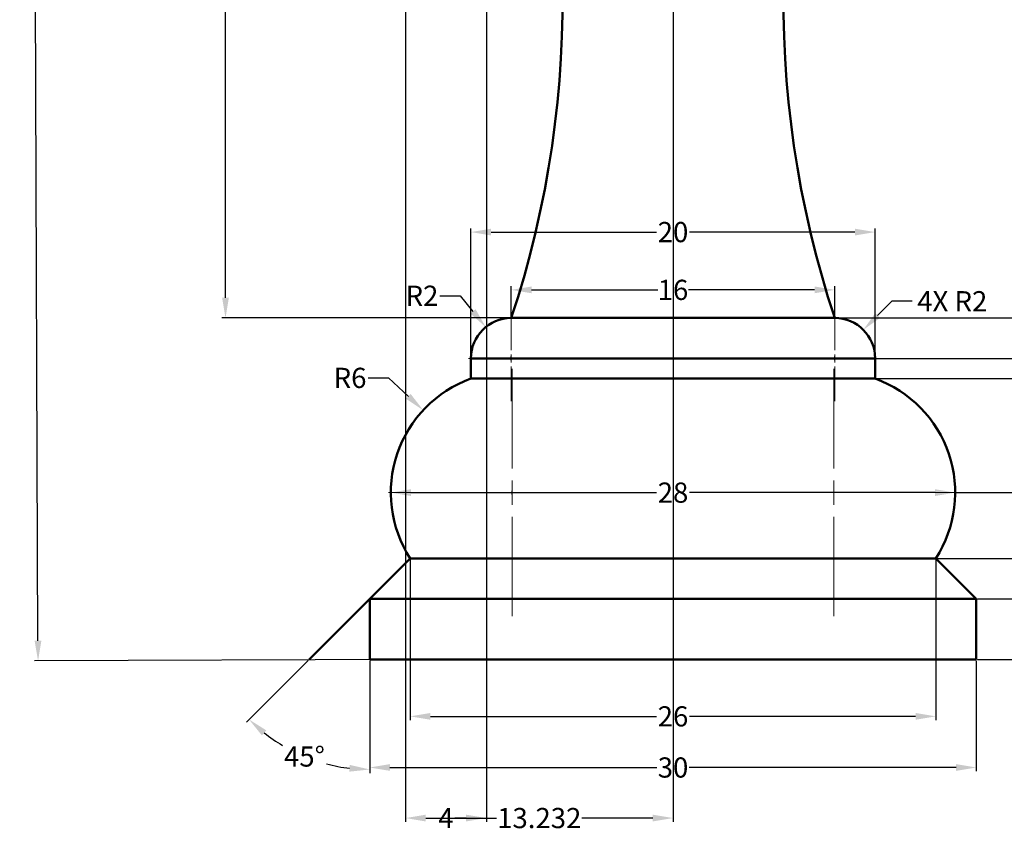
# Model space of a CAD drawing. Units: millimetres. Extents: x 31 to 232, y 35 to 192.
# Tile 1 of 5: x 31 to 80, y 35 to 75. Entities that reach past the tile are written whole.
import ezdxf

# ---------------------------------------------------------------- set-up
doc = ezdxf.new("R2010")
doc.units = ezdxf.units.MM
doc.header["$MEASUREMENT"] = 0
doc.linetypes.add('CENTER', pattern=[50.8, 31.75, -6.35, 6.35, -6.35])
for name, color, linetype, lineweight in [('M-CNTR', 1, 'CENTER', 18), ('M-DIMS', 2, 'Continuous', 25), ('M-OUTL', 7, 'Continuous', 50)]:
    doc.layers.add(name, color=color, linetype=linetype, lineweight=lineweight)
doc.styles.get("Standard").update_dxf_attribs({"font": 'arial.ttf'})
doc.dimstyles.get("Standard").update_dxf_attribs({"dimtxt": 1, "dimasz": 1, "dimexe": 0.18, "dimexo": 0.0625, "dimgap": 0.09, "dimtad": 0, "dimtih": 1, "dimtoh": 1, "dimdec": 0, "dimzin": 0, "dimdsep": 46, "dimtxsty": 'Standard', "dimcen": 0.09, "dimadec": 0, "dimazin": 0, "dimtfac": 1, "dimtdec": 0, "dimtofl": 0, "dimtmove": 0, "dimatfit": 3, "dimfxl": 1, "dimtolj": 1, "dimtzin": 0, "dimarcsym": 0})

# ---------------------------------------------------------------- blocks, each defined once
blk = doc.blocks.new('*D1')
at = {"layer": 'Defpoints', "color": 0, "transparency": 16777216}
for p in [(50.774, 48.183), (48.774, 46.183), (45.774, 43.183), (48.774, 43.183), (44.551, 38.869)]:
    blk.add_point(p, dxfattribs=at)
at = {"layer": 'M-DIMS', "color": 0, "lineweight": -2, "transparency": 16777216}
for p, q in [((45.729, 43.139), (42.674, 40.084)), ((48.774, 43.12), (48.774, 37.557))]:
    blk.add_line(p, q, dxfattribs=at)
for start, end in [(231.788, 239.2119), (255.3151, 263.212)]:
    blk.add_arc((48.774, 46.183), 8.446, start, end, dxfattribs=at)
at = {"layer": 'M-DIMS', "color": 0, "transparency": 16777216}
for points in [[(43.439, 39.422), (43.66, 39.671), (42.802, 40.211)], [(47.785, 37.963), (47.765, 37.63), (48.774, 37.737)]]:
    blk.add_solid(points, dxfattribs=at)
at = {"layer": 'M-DIMS', "color": 0, "transparency": 16777216, "insert": (45.542, 38.38), "char_height": 1, "attachment_point": 5}
blk.add_mtext('\\A1;45°', dxfattribs=at)
blk = doc.blocks.new('*D2')
at = {"layer": 'Defpoints', "color": 0, "transparency": 16777216}
for p in [(51.415, 55.522), (55.813, 51.44)]:
    blk.add_point(p, dxfattribs=at)
at = {"layer": 'M-DIMS', "color": 0, "lineweight": -2, "transparency": 16777216}
for p, q in [((48.694, 57.119), (49.694, 57.119)), ((49.694, 57.119), (50.682, 56.202)), ((55.723, 51.44), (55.903, 51.44)), ((55.813, 51.35), (55.813, 51.53))]:
    blk.add_line(p, q, dxfattribs=at)
at = {"layer": 'M-DIMS', "color": 0, "transparency": 16777216}
blk.add_solid([(50.795, 56.324), (50.568, 56.08), (51.415, 55.522)], dxfattribs=at)
at = {"layer": 'M-DIMS', "color": 0, "transparency": 16777216, "insert": (47.798, 57.119), "char_height": 1, "attachment_point": 5}
blk.add_mtext('\\A1;R6', dxfattribs=at)
blk = doc.blocks.new('*D3')
at = {"layer": 'Defpoints', "color": 0, "transparency": 16777216}
for p in [(54.51, 59.633), (55.774, 58.083)]:
    blk.add_point(p, dxfattribs=at)
at = {"layer": 'M-DIMS', "color": 0, "lineweight": -2, "transparency": 16777216}
for p, q in [((52.247, 61.184), (53.247, 61.184)), ((53.247, 61.184), (53.878, 60.408)), ((55.684, 58.083), (55.864, 58.083)), ((55.774, 57.993), (55.774, 58.173))]:
    blk.add_line(p, q, dxfattribs=at)
at = {"layer": 'M-DIMS', "color": 0, "transparency": 16777216}
blk.add_solid([(54.008, 60.514), (53.749, 60.303), (54.51, 59.633)], dxfattribs=at)
at = {"layer": 'M-DIMS', "color": 0, "transparency": 16777216, "insert": (51.356, 61.184), "char_height": 1, "attachment_point": 5}
blk.add_mtext('\\A1;R2', dxfattribs=at)
blk = doc.blocks.new('*D4')
at = {"layer": 'Defpoints', "color": 0, "transparency": 16777216}
for p in [(78.774, 46.183), (119.423, 46.183), (78.774, 43.183)]:
    blk.add_point(p, dxfattribs=at)
at = {"layer": 'M-DIMS', "color": 0, "lineweight": -2, "transparency": 16777216}
for p, q in [((119.423, 46.183), (119.423, 47.183)), ((119.423, 47.183), (120.423, 47.183)), ((78.836, 46.183), (119.603, 46.183)), ((119.423, 44.183), (119.423, 45.183)), ((78.836, 43.183), (119.603, 43.183))]:
    blk.add_line(p, q, dxfattribs=at)
at = {"layer": 'M-DIMS', "color": 0, "transparency": 16777216}
for points in [[(119.256, 45.183), (119.589, 45.183), (119.423, 46.183)], [(119.256, 44.183), (119.589, 44.183), (119.423, 43.183)]]:
    blk.add_solid(points, dxfattribs=at)
at = {"layer": 'M-DIMS', "color": 0, "transparency": 16777216, "insert": (120.84, 47.183), "char_height": 1, "attachment_point": 5}
blk.add_mtext('\\A1;3', dxfattribs=at)
blk = doc.blocks.new('*D5')
at = {"layer": 'Defpoints', "color": 0, "transparency": 16777216}
for p in [(76.774, 48.183), (119.423, 48.183), (78.774, 46.183)]:
    blk.add_point(p, dxfattribs=at)
at = {"layer": 'M-DIMS', "color": 0, "lineweight": -2, "transparency": 16777216}
for p, q in [((119.423, 49.183), (119.423, 50.183)), ((76.836, 48.183), (119.603, 48.183)), ((78.836, 46.183), (119.603, 46.183)), ((119.423, 45.183), (119.423, 44.183))]:
    blk.add_line(p, q, dxfattribs=at)
at = {"layer": 'M-DIMS', "color": 0, "transparency": 16777216}
for points in [[(119.256, 49.183), (119.589, 49.183), (119.423, 48.183)], [(119.256, 45.183), (119.589, 45.183), (119.423, 46.183)]]:
    blk.add_solid(points, dxfattribs=at)
at = {"layer": 'M-DIMS', "color": 0, "transparency": 16777216, "insert": (119.423, 47.183), "char_height": 1, "attachment_point": 5}
blk.add_mtext('\\A1;2', dxfattribs=at)
blk = doc.blocks.new('*D6')
at = {"layer": 'Defpoints', "color": 0, "transparency": 16777216}
for p in [(77.735, 51.44), (119.423, 51.44), (76.774, 48.183)]:
    blk.add_point(p, dxfattribs=at)
at = {"layer": 'M-DIMS', "color": 0, "lineweight": -2, "transparency": 16777216}
for p, q in [((119.423, 51.44), (119.423, 52.44)), ((119.423, 52.44), (120.423, 52.44)), ((77.797, 51.44), (119.603, 51.44)), ((119.423, 49.183), (119.423, 50.44)), ((76.836, 48.183), (119.603, 48.183))]:
    blk.add_line(p, q, dxfattribs=at)
at = {"layer": 'M-DIMS', "color": 0, "transparency": 16777216}
for points in [[(119.256, 50.44), (119.589, 50.44), (119.423, 51.44)], [(119.256, 49.183), (119.589, 49.183), (119.423, 48.183)]]:
    blk.add_solid(points, dxfattribs=at)
at = {"layer": 'M-DIMS', "color": 0, "transparency": 16777216, "insert": (120.84, 52.44), "char_height": 1, "attachment_point": 5}
blk.add_mtext('\\A1;3', dxfattribs=at)
blk = doc.blocks.new('*D7')
at = {"layer": 'Defpoints', "color": 0, "transparency": 16777216}
for p in [(73.774, 57.083), (119.423, 57.083), (77.735, 51.44)]:
    blk.add_point(p, dxfattribs=at)
at = {"layer": 'M-DIMS', "color": 0, "lineweight": -2, "transparency": 16777216}
for p, q in [((73.836, 57.083), (119.603, 57.083)), ((119.423, 56.083), (119.423, 54.862)), ((119.423, 52.44), (119.423, 53.661)), ((77.797, 51.44), (119.603, 51.44))]:
    blk.add_line(p, q, dxfattribs=at)
at = {"layer": 'M-DIMS', "color": 0, "transparency": 16777216}
for points in [[(119.256, 56.083), (119.589, 56.083), (119.423, 57.083)], [(119.256, 52.44), (119.589, 52.44), (119.423, 51.44)]]:
    blk.add_solid(points, dxfattribs=at)
at = {"layer": 'M-DIMS', "color": 0, "transparency": 16777216, "insert": (119.423, 54.261), "char_height": 1, "attachment_point": 5}
blk.add_mtext('\\A1;6', dxfattribs=at)
blk = doc.blocks.new('*D8')
at = {"layer": 'Defpoints', "color": 0, "transparency": 16777216}
for p in [(73.774, 58.083), (119.423, 58.083), (73.774, 57.083)]:
    blk.add_point(p, dxfattribs=at)
at = {"layer": 'M-DIMS', "color": 0, "lineweight": -2, "transparency": 16777216}
for p, q in [((119.423, 59.083), (119.423, 60.083)), ((119.423, 60.083), (120.423, 60.083)), ((73.836, 58.083), (119.603, 58.083)), ((73.836, 57.083), (119.603, 57.083)), ((119.423, 56.083), (119.423, 55.083))]:
    blk.add_line(p, q, dxfattribs=at)
at = {"layer": 'M-DIMS', "color": 0, "transparency": 16777216}
for points in [[(119.256, 59.083), (119.589, 59.083), (119.423, 58.083)], [(119.256, 56.083), (119.589, 56.083), (119.423, 57.083)]]:
    blk.add_solid(points, dxfattribs=at)
at = {"layer": 'M-DIMS', "color": 0, "transparency": 16777216, "insert": (120.697, 60.083), "char_height": 1, "attachment_point": 5}
blk.add_mtext('\\A1;1', dxfattribs=at)
blk = doc.blocks.new('*D9')
at = {"layer": 'Defpoints', "color": 0, "transparency": 16777216}
for p in [(71.774, 60.083), (119.423, 60.083), (73.774, 58.083)]:
    blk.add_point(p, dxfattribs=at)
at = {"layer": 'M-DIMS', "color": 0, "lineweight": -2, "transparency": 16777216}
for p, q in [((119.423, 61.083), (119.423, 62.083)), ((71.836, 60.083), (119.603, 60.083)), ((73.836, 58.083), (119.603, 58.083)), ((119.423, 57.083), (119.423, 56.083))]:
    blk.add_line(p, q, dxfattribs=at)
at = {"layer": 'M-DIMS', "color": 0, "transparency": 16777216}
for points in [[(119.256, 61.083), (119.589, 61.083), (119.423, 60.083)], [(119.256, 57.083), (119.589, 57.083), (119.423, 58.083)]]:
    blk.add_solid(points, dxfattribs=at)
at = {"layer": 'M-DIMS', "color": 0, "transparency": 16777216, "insert": (119.423, 59.083), "char_height": 1, "attachment_point": 5}
blk.add_mtext('\\A1;2', dxfattribs=at)
blk = doc.blocks.new('*D10')
at = {"layer": 'Defpoints', "color": 0, "transparency": 16777216}
for p in [(119.236, 75.81), (119.423, 75.81), (71.774, 60.083)]:
    blk.add_point(p, dxfattribs=at)
at = {"layer": 'M-DIMS', "color": 0, "lineweight": -2, "transparency": 16777216}
for p, q in [((119.298, 75.81), (119.603, 75.81)), ((119.423, 74.81), (119.423, 68.547)), ((119.423, 61.083), (119.423, 67.346)), ((71.836, 60.083), (119.603, 60.083))]:
    blk.add_line(p, q, dxfattribs=at)
at = {"layer": 'M-DIMS', "color": 0, "transparency": 16777216}
for points in [[(119.256, 74.81), (119.589, 74.81), (119.423, 75.81)], [(119.256, 61.083), (119.589, 61.083), (119.423, 60.083)]]:
    blk.add_solid(points, dxfattribs=at)
at = {"layer": 'M-DIMS', "color": 0, "transparency": 16777216, "insert": (119.423, 67.946), "char_height": 1, "attachment_point": 5}
blk.add_mtext('\\A1;16', dxfattribs=at)
blk = doc.blocks.new('*D18')
at = {"layer": 'Defpoints', "color": 0, "transparency": 16777216}
for p in [(48.774, 43.183), (78.774, 43.183), (78.774, 37.835)]:
    blk.add_point(p, dxfattribs=at)
at = {"layer": 'M-DIMS', "color": 0, "lineweight": -2, "transparency": 16777216}
for p, q in [((48.774, 43.12), (48.774, 37.655)), ((78.774, 43.12), (78.774, 37.655)), ((49.774, 37.835), (62.969, 37.835)), ((77.774, 37.835), (64.578, 37.835))]:
    blk.add_line(p, q, dxfattribs=at)
at = {"layer": 'M-DIMS', "color": 0, "transparency": 16777216}
for points in [[(49.774, 38.002), (49.774, 37.669), (48.774, 37.835)], [(77.774, 38.002), (77.774, 37.669), (78.774, 37.835)]]:
    blk.add_solid(points, dxfattribs=at)
at = {"layer": 'M-DIMS', "color": 0, "transparency": 16777216, "insert": (63.774, 37.835), "char_height": 1, "attachment_point": 5}
blk.add_mtext('\\A1;30', dxfattribs=at)
blk = doc.blocks.new('*D19')
at = {"layer": 'Defpoints', "color": 0, "transparency": 16777216}
for p in [(50.774, 48.183), (76.774, 48.183), (76.774, 40.366)]:
    blk.add_point(p, dxfattribs=at)
at = {"layer": 'M-DIMS', "color": 0, "lineweight": -2, "transparency": 16777216}
for p, q in [((50.774, 48.12), (50.774, 40.186)), ((76.774, 48.12), (76.774, 40.186)), ((51.774, 40.366), (62.959, 40.366)), ((75.774, 40.366), (64.588, 40.366))]:
    blk.add_line(p, q, dxfattribs=at)
at = {"layer": 'M-DIMS', "color": 0, "transparency": 16777216}
for points in [[(51.774, 40.533), (51.774, 40.199), (50.774, 40.366)], [(75.774, 40.533), (75.774, 40.199), (76.774, 40.366)]]:
    blk.add_solid(points, dxfattribs=at)
at = {"layer": 'M-DIMS', "color": 0, "transparency": 16777216, "insert": (63.774, 40.366), "char_height": 1, "attachment_point": 5}
blk.add_mtext('\\A1;26', dxfattribs=at)
blk = doc.blocks.new('*D20')
at = {"layer": 'Defpoints', "color": 0, "transparency": 16777216}
for p in [(49.813, 51.44), (77.735, 51.44), (77.735, 51.44)]:
    blk.add_point(p, dxfattribs=at)
at = {"layer": 'M-DIMS', "color": 0, "lineweight": -2, "transparency": 16777216}
for p, q in [((49.813, 51.502), (49.813, 51.62)), ((50.813, 51.44), (62.958, 51.44)), ((76.735, 51.44), (64.589, 51.44)), ((77.735, 51.502), (77.735, 51.62))]:
    blk.add_line(p, q, dxfattribs=at)
at = {"layer": 'M-DIMS', "color": 0, "transparency": 16777216}
for points in [[(50.813, 51.607), (50.813, 51.273), (49.813, 51.44)], [(76.735, 51.607), (76.735, 51.273), (77.735, 51.44)]]:
    blk.add_solid(points, dxfattribs=at)
at = {"layer": 'M-DIMS', "color": 0, "transparency": 16777216, "insert": (63.774, 51.44), "char_height": 1, "attachment_point": 5}
blk.add_mtext('\\A1;28', dxfattribs=at)
blk = doc.blocks.new('*D21')
at = {"layer": 'Defpoints', "color": 0, "transparency": 16777216}
for p in [(73.774, 64.335), (53.774, 57.083), (73.774, 57.083)]:
    blk.add_point(p, dxfattribs=at)
at = {"layer": 'M-DIMS', "color": 0, "lineweight": -2, "transparency": 16777216}
for p, q in [((53.774, 57.145), (53.774, 64.515)), ((54.774, 64.335), (62.961, 64.335)), ((72.774, 64.335), (64.587, 64.335)), ((73.774, 57.145), (73.774, 64.515))]:
    blk.add_line(p, q, dxfattribs=at)
at = {"layer": 'M-DIMS', "color": 0, "transparency": 16777216}
for points in [[(54.774, 64.501), (54.774, 64.168), (53.774, 64.335)], [(72.774, 64.501), (72.774, 64.168), (73.774, 64.335)]]:
    blk.add_solid(points, dxfattribs=at)
at = {"layer": 'M-DIMS', "color": 0, "transparency": 16777216, "insert": (63.774, 64.335), "char_height": 1, "attachment_point": 5}
blk.add_mtext('\\A1;20', dxfattribs=at)
blk = doc.blocks.new('*D22')
at = {"layer": 'Defpoints', "color": 0, "transparency": 16777216}
for p in [(71.774, 61.474), (55.774, 60.083), (71.774, 60.083)]:
    blk.add_point(p, dxfattribs=at)
at = {"layer": 'M-DIMS', "color": 0, "lineweight": -2, "transparency": 16777216}
for p, q in [((55.774, 60.145), (55.774, 61.654)), ((56.774, 61.474), (63.015, 61.474)), ((70.774, 61.474), (64.532, 61.474)), ((71.774, 60.145), (71.774, 61.654))]:
    blk.add_line(p, q, dxfattribs=at)
at = {"layer": 'M-DIMS', "color": 0, "transparency": 16777216}
for points in [[(56.774, 61.641), (56.774, 61.307), (55.774, 61.474)], [(70.774, 61.641), (70.774, 61.307), (71.774, 61.474)]]:
    blk.add_solid(points, dxfattribs=at)
at = {"layer": 'M-DIMS', "color": 0, "transparency": 16777216, "insert": (63.774, 61.474), "char_height": 1, "attachment_point": 5}
blk.add_mtext('\\A1;16', dxfattribs=at)
blk = doc.blocks.new('*D24')
at = {"layer": 'Defpoints', "color": 0, "transparency": 16777216}
for p in [(32.062, 118.008), (50.471, 118.083), (50.774, 43.183)]:
    blk.add_point(p, dxfattribs=at)
at = {"layer": 'M-DIMS', "color": 0, "lineweight": -2, "transparency": 16777216}
for p, q in [((50.408, 118.083), (31.882, 118.008)), ((32.066, 117.008), (32.211, 81.157)), ((32.361, 44.108), (32.216, 79.96)), ((50.711, 43.183), (32.185, 43.108))]:
    blk.add_line(p, q, dxfattribs=at)
at = {"layer": 'M-DIMS', "color": 0, "transparency": 16777216}
for points in [[(32.233, 117.009), (31.9, 117.008), (32.062, 118.008)], [(32.528, 44.109), (32.195, 44.108), (32.365, 43.108)]]:
    blk.add_solid(points, dxfattribs=at)
at = {"layer": 'M-DIMS', "color": 0, "transparency": 16777216, "insert": (32.214, 80.558), "char_height": 1, "attachment_point": 5}
blk.add_mtext('\\A1;75', dxfattribs=at)
blk = doc.blocks.new('*D30')
at = {"layer": 'Defpoints', "color": 0, "transparency": 16777216}
for p in [(41.638, 94.283), (63.774, 94.283), (63.774, 60.083)]:
    blk.add_point(p, dxfattribs=at)
at = {"layer": 'M-DIMS', "color": 0, "lineweight": -2, "transparency": 16777216}
for p, q in [((63.711, 94.283), (41.458, 94.283)), ((41.638, 93.283), (41.638, 77.784)), ((41.638, 61.083), (41.638, 76.582)), ((63.711, 60.083), (41.458, 60.083))]:
    blk.add_line(p, q, dxfattribs=at)
at = {"layer": 'M-DIMS', "color": 0, "transparency": 16777216}
for points in [[(41.471, 93.283), (41.805, 93.283), (41.638, 94.283)], [(41.471, 61.083), (41.805, 61.083), (41.638, 60.083)]]:
    blk.add_solid(points, dxfattribs=at)
at = {"layer": 'M-DIMS', "color": 0, "transparency": 16777216, "insert": (41.638, 77.183), "char_height": 1, "attachment_point": 5}
blk.add_mtext('\\A1;34', dxfattribs=at)
blk = doc.blocks.new('*U35')
at = {"layer": 'M-CNTR', "color": 0, "transparency": 16777216}
for p, q in [((0, 0.4), (0, 2.12)), ((-2.12, 0), (-0.4, 0)), ((0.4, 0), (2.12, 0)), ((0, -2.12), (0, -0.4))]:
    blk.add_line(p, q, dxfattribs=at)
at = {"layer": 'M-CNTR', "color": 0, "linetype": 'Continuous', "transparency": 16777216}
for p, q in [((-0.2, 0), (0.2, 0)), ((0, -0.2), (0, 0.2))]:
    blk.add_line(p, q, dxfattribs=at)
blk = doc.blocks.new('*U36')
at = {"layer": 'M-CNTR', "color": 0, "transparency": 16777216}
for p, q in [((0, 0.4), (0, 2.12)), ((-2.12, 0), (-0.4, 0)), ((0.4, 0), (2.12, 0)), ((0, -2.12), (0, -0.4))]:
    blk.add_line(p, q, dxfattribs=at)
at = {"layer": 'M-CNTR', "color": 0, "linetype": 'Continuous', "transparency": 16777216}
for p, q in [((-0.2, 0), (0.2, 0)), ((0, -0.2), (0, 0.2))]:
    blk.add_line(p, q, dxfattribs=at)
blk = doc.blocks.new('*U37')
at = {"layer": 'M-CNTR', "color": 0, "transparency": 16777216}
for p, q in [((0, 1.2), (0, 6.12)), ((-6.12, 0), (-1.2, 0)), ((1.2, 0), (6.12, 0)), ((0, -6.12), (0, -1.2))]:
    blk.add_line(p, q, dxfattribs=at)
at = {"layer": 'M-CNTR', "color": 0, "linetype": 'Continuous', "transparency": 16777216}
for p, q in [((0, -0.6), (0, 0.6)), ((-0.6, 0), (0.6, 0))]:
    blk.add_line(p, q, dxfattribs=at)
blk = doc.blocks.new('*U38')
at = {"layer": 'M-CNTR', "color": 0, "transparency": 16777216}
for p, q in [((0, 1.2), (0, 6.12)), ((-6.12, 0), (-1.2, 0)), ((1.2, 0), (6.12, 0)), ((0, -6.12), (0, -1.2))]:
    blk.add_line(p, q, dxfattribs=at)
at = {"layer": 'M-CNTR', "color": 0, "linetype": 'Continuous', "transparency": 16777216}
for p, q in [((0, -0.6), (0, 0.6)), ((-0.6, 0), (0.6, 0))]:
    blk.add_line(p, q, dxfattribs=at)
blk = doc.blocks.new('*D43')
at = {"layer": 'Defpoints', "color": 0, "transparency": 16777216}
for p in [(50.542, 106.433), (63.774, 106.433), (63.774, 35.333)]:
    blk.add_point(p, dxfattribs=at)
at = {"layer": 'M-DIMS', "color": 0, "lineweight": -2, "transparency": 16777216}
for p, q in [((50.542, 106.37), (50.542, 35.153)), ((63.774, 106.37), (63.774, 35.153)), ((51.542, 35.333), (55.044, 35.333)), ((62.774, 35.333), (59.271, 35.333))]:
    blk.add_line(p, q, dxfattribs=at)
at = {"layer": 'M-DIMS', "color": 0, "transparency": 16777216}
for points in [[(51.542, 35.5), (51.542, 35.166), (50.542, 35.333)], [(62.774, 35.5), (62.774, 35.166), (63.774, 35.333)]]:
    blk.add_solid(points, dxfattribs=at)
at = {"layer": 'M-DIMS', "color": 0, "transparency": 16777216, "insert": (57.158, 35.333), "char_height": 1, "attachment_point": 5}
blk.add_mtext('\\A1;13.232', dxfattribs=at)
blk = doc.blocks.new('*D44')
at = {"layer": 'Defpoints', "color": 0, "transparency": 16777216}
for p in [(50.542, 113.083), (54.542, 110.083), (54.542, 35.333)]:
    blk.add_point(p, dxfattribs=at)
at = {"layer": 'M-DIMS', "color": 0, "lineweight": -2, "transparency": 16777216}
for p, q in [((50.542, 113.02), (50.542, 35.153)), ((54.542, 110.02), (54.542, 35.153)), ((51.542, 35.333), (52.106, 35.333)), ((53.542, 35.333), (52.977, 35.333))]:
    blk.add_line(p, q, dxfattribs=at)
at = {"layer": 'M-DIMS', "color": 0, "transparency": 16777216}
for points in [[(51.542, 35.5), (51.542, 35.166), (50.542, 35.333)], [(53.542, 35.5), (53.542, 35.166), (54.542, 35.333)]]:
    blk.add_solid(points, dxfattribs=at)
at = {"layer": 'M-DIMS', "color": 0, "transparency": 16777216, "insert": (52.542, 35.333), "char_height": 1, "attachment_point": 5}
blk.add_mtext('\\A1;4', dxfattribs=at)
blk = doc.blocks.new('*D47')
at = {"layer": 'Defpoints', "color": 0, "transparency": 16777216}
for p in [(73.188, 59.497), (71.774, 58.083)]:
    blk.add_point(p, dxfattribs=at)
at = {"layer": 'M-DIMS', "color": 0, "lineweight": -2, "transparency": 16777216}
for p, q in [((74.602, 60.911), (73.895, 60.204)), ((75.602, 60.911), (74.602, 60.911)), ((71.684, 58.083), (71.864, 58.083)), ((71.774, 57.993), (71.774, 58.173))]:
    blk.add_line(p, q, dxfattribs=at)
at = {"layer": 'M-DIMS', "color": 0, "transparency": 16777216}
blk.add_solid([(73.777, 60.322), (74.013, 60.086), (73.188, 59.497)], dxfattribs=at)
at = {"layer": 'M-DIMS', "color": 0, "transparency": 16777216, "insert": (77.588, 60.911), "char_height": 1, "attachment_point": 5}
blk.add_mtext('\\A1;4X R2', dxfattribs=at)

msp = doc.modelspace()

# ---------------------------------------------------------------- linework, layer by layer
at = {"layer": 'M-OUTL'}
for p, q in [((55.7736, 60.0829), (63.7736, 60.0829)), ((71.7736, 60.0829), (63.7736, 60.0829)), ((53.7736, 57.0829), (53.7736, 58.0829)), ((53.7736, 58.0829), (63.7736, 58.0829)), ((73.7736, 58.0829), (63.7736, 58.0829)), ((73.7736, 57.0829), (73.7736, 58.0829)), ((63.7736, 57.0829), (53.7736, 57.0829)), ((63.7736, 57.0829), (73.7736, 57.0829)), ((50.7736, 48.1829), (45.7736, 43.1829)), ((63.7736, 48.1829), (50.7736, 48.1829)), ((63.7736, 48.1829), (76.7736, 48.1829)), ((76.7736, 48.1829), (78.7736, 46.1829)), ((78.7736, 46.1829), (48.7736, 46.1829)), ((48.7736, 46.1829), (48.7736, 43.1829)), ((78.7736, 43.1829), (78.7736, 46.1829)), ((78.7736, 46.1829), (78.7736, 43.1829)), ((48.7736, 43.1829), (78.7736, 43.1829))]:
    msp.add_line(p, q, dxfattribs=at)
for centre, radius, start, end in [((8.3113, 75.8097), 50, 341.66715, 21.68252), ((119.2359, 75.8097), 50, 158.31748, 198.33285), ((55.7736, 58.0829), 2, 90, 180), ((71.7736, 58.0829), 2, 0, 90), ((55.8126, 51.44), 6, 109.86661, 212.87766), ((71.7346, 51.44), 6, 327.12234, 70.13339)]:
    msp.add_arc(centre, radius, start, end, dxfattribs=at)

# ---------------------------------------------------------------- block references
at = {"layer": 'M-CNTR'}
for name, p in [('*U36', (55.7736, 58.0829)), ('*U35', (71.7736, 58.0829)), ('*U38', (55.8126, 51.44)), ('*U37', (71.7346, 51.44))]:
    msp.add_blockref(name, p, dxfattribs=at)

# ---------------------------------------------------------------- dimensions: what is measured, and where the dimension line sits
at = {"layer": 'M-DIMS'}
dim = msp.add_aligned_dim(p1=(50.7736, 43.1829), p2=(50.4706, 118.0829), distance=18.4084, dimstyle='Standard', override={"dimclrd": 0, "dimclre": 0, "dimclrt": 0}, dxfattribs=at)
dim.commit()
dim.dimension.update_dxf_attribs({"geometry": '*D24', "text_midpoint": (32.2138, 80.5584)})
for base, p1, p2, override, picture, middle in [((54.5416, 35.3329), (50.5416, 113.0829), (54.5416, 110.0829), {"dimdec": 0, "dimlfac": 1, "dimrnd": 0, "dimzin": 0, "dimdsep": 46, "dimlunit": 2}, '*D44', (52.5416, 35.3329)), ((63.7736, 35.3329), (50.5416, 106.4329), (63.7736, 106.4329), {"dimdec": 3, "dimlfac": 1, "dimrnd": 0, "dimzin": 0, "dimdsep": 46, "dimlunit": 2}, '*D43', (57.1576, 35.3329)), ((73.7736, 64.3346), (53.7736, 57.0829), (73.7736, 57.0829), {"dimclrd": 0, "dimclre": 0, "dimclrt": 0}, '*D21', (63.7736, 64.3346)), ((71.7736, 61.4739), (55.7736, 60.0829), (71.7736, 60.0829), {"dimclrd": 0, "dimclre": 0, "dimclrt": 0}, '*D22', (63.7736, 61.4739)), ((77.7346, 51.44), (49.8126, 51.44), (77.7346, 51.44), {"dimclrd": 0, "dimclre": 0, "dimclrt": 0}, '*D20', (63.7736, 51.44)), ((76.7736, 40.3661), (50.7736, 48.1829), (76.7736, 48.1829), {"dimclrd": 0, "dimclre": 0, "dimclrt": 0}, '*D19', (63.7736, 40.3661)), ((78.7736, 37.8352), (48.7736, 43.1829), (78.7736, 43.1829), {"dimclrd": 0, "dimclre": 0, "dimclrt": 0}, '*D18', (63.7736, 37.8352))]:
    dim = msp.add_linear_dim(base=base, p1=p1, p2=p2, dimstyle='Standard', override=override, dxfattribs=at)
    dim.commit()
    dim.dimension.update_dxf_attribs({"geometry": picture, "text_midpoint": middle})
for base, p1, p2, angle, picture, middle in [((41.6381, 94.2829), (63.7736, 60.0829), (63.7736, 94.2829), 90, '*D30', (41.6381, 77.1829)), ((119.4225, 75.8097), (71.7736, 60.0829), (119.2359, 75.8097), 270, '*D10', (119.4225, 67.9463)), ((119.4225, 60.0829), (73.7736, 58.0829), (71.7736, 60.0829), 270, '*D9', (119.4225, 59.0829)), ((119.4225, 58.0829), (73.7736, 57.0829), (73.7736, 58.0829), 270, '*D8', (120.6967, 60.0829)), ((119.4225, 57.0829), (77.7346, 51.44), (73.7736, 57.0829), 270, '*D7', (119.4225, 54.2614)), ((119.4225, 51.44), (76.7736, 48.1829), (77.7346, 51.44), 270, '*D6', (120.8399, 52.44)), ((119.4225, 48.1829), (78.7736, 46.1829), (76.7736, 48.1829), 270, '*D5', (119.4225, 47.1829)), ((119.4225, 46.1829), (78.7736, 43.1829), (78.7736, 46.1829), 270, '*D4', (120.8399, 47.1829))]:
    dim = msp.add_linear_dim(base=base, p1=p1, p2=p2, angle=angle, dimstyle='Standard', override={"dimclrd": 0, "dimclre": 0, "dimclrt": 0}, dxfattribs=at)
    dim.commit()
    dim.dimension.update_dxf_attribs({"geometry": picture, "text_midpoint": middle})
dim = msp.add_radius_dim(center=(71.7736, 58.0829), mpoint=(73.188, 59.497), text='4X <>', dimstyle='Standard', override={"dimdec": 0, "dimlfac": 1, "dimrnd": 0, "dimzin": 0, "dimdsep": 46, "dimlunit": 2}, dxfattribs=at)
dim.commit()
dim.dimension.update_dxf_attribs({"geometry": '*D47', "text_midpoint": (77.5879, 60.911)})
dim = msp.add_radius_dim(center=(55.7736, 58.0829), mpoint=(54.5102, 59.6333), dimstyle='Standard', override={"dimclrd": 0, "dimclre": 0, "dimclrt": 0}, dxfattribs=at)
dim.commit()
dim.dimension.update_dxf_attribs({"geometry": '*D3', "text_midpoint": (51.3556, 61.1837)})
dim = msp.add_radius_dim(center=(55.8126, 51.44), mpoint=(51.4148, 55.5216), dimstyle='Standard', override={"dimclrd": 0, "dimclre": 0, "dimclrt": 0}, dxfattribs=at)
dim.commit()
dim.dimension.update_dxf_attribs({"geometry": '*D2', "text_midpoint": (47.798, 57.1188), "dimtype": 164})
dim = msp.add_angular_dim_2l(base=(44.5507, 38.8687), line1=((48.7736, 46.1829), (48.7736, 43.1829)), line2=((50.7736, 48.1829), (45.7736, 43.1829)), dimstyle='Standard', override={"dimclrd": 0, "dimclre": 0, "dimclrt": 0}, dxfattribs=at)
dim.commit()
dim.dimension.update_dxf_attribs({"geometry": '*D1', "text_midpoint": (45.5416, 38.3801)})

doc.saveas('drawing.dxf')
